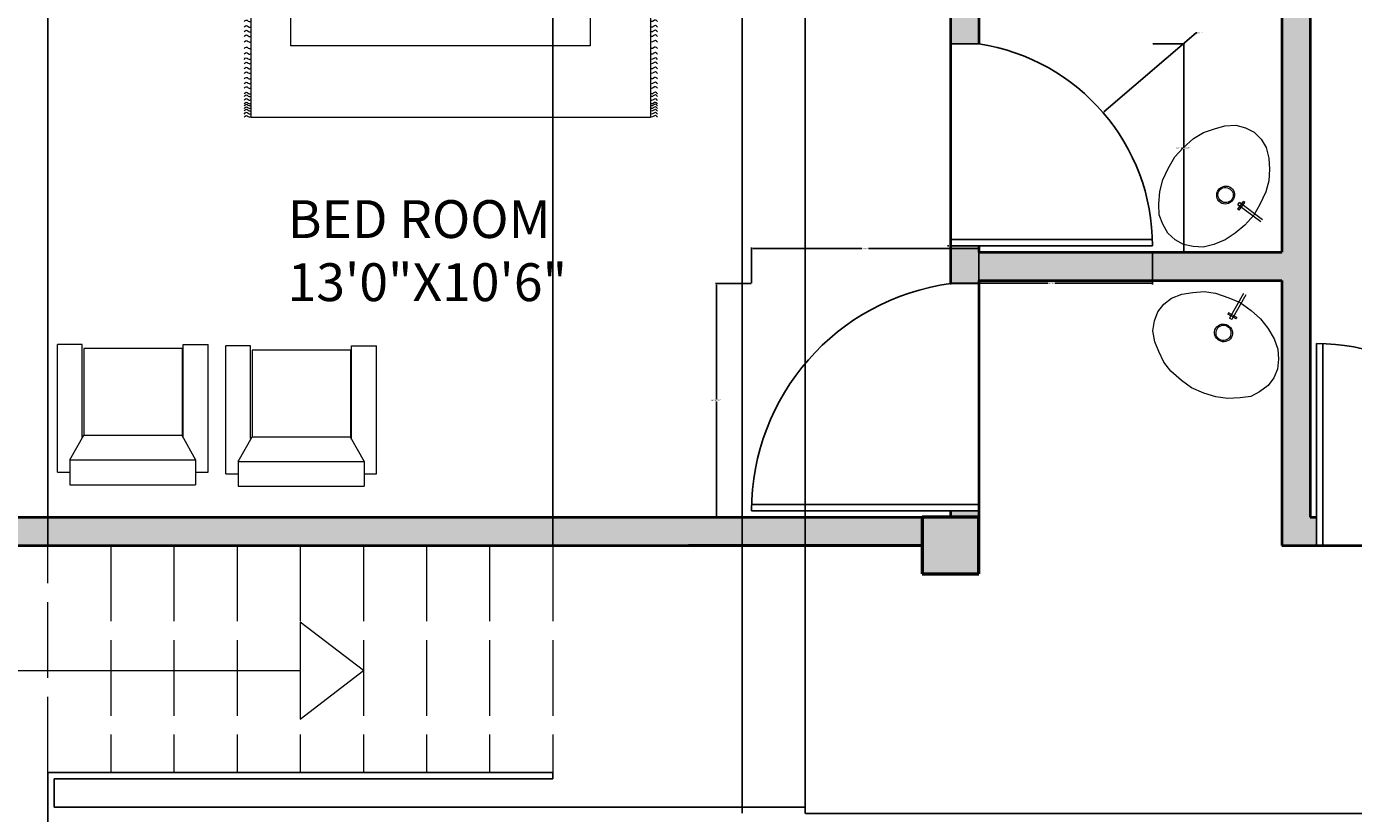
# Model space of a CAD drawing. Units: inches. Extents: x 25176543 to 25177243, y 80295576 to 80296086.
# Tile 3 of 11: x 25176668 to 25176879, y 80295843 to 80295968. Entities that reach past the tile are written whole.
import ezdxf

# ---------------------------------------------------------------- set-up
doc = ezdxf.new("R2010")
doc.units = ezdxf.units.IN
doc.header["$MEASUREMENT"] = 0
doc.linetypes.add('ACAD_ISO02W100', pattern=[15, 12, -3])
for name, color, linetype, lineweight in [('A-ANNO-DIMS', 2, 'Continuous', 18), ('A-ANNO-SYMB', 7, 'Continuous', 18), ('A-AREA-IDEN', 7, 'Continuous', 18), ('A-COLS', 7, 'Continuous', 50), ('A-COLS-PATT', 251, 'Continuous', 13), ('A-DOOR', 3, 'Continuous', 25), ('A-FLOR-FIXT', 8, 'Continuous', 18), ('A-FLOR-STRS', 7, 'Continuous', 25), ('A-FLOR-STRS-OVHD', 7, 'ACAD_ISO02W100', 18), ('A-WALL', 7, 'Continuous', 40), ('A-WALL-PATT', 146, 'Continuous', 13), ('furniture', 31, 'Continuous', 13)]:
    doc.layers.add(name, color=color, linetype=linetype, lineweight=lineweight)
doc.styles.get("Standard").update_dxf_attribs({"font": 'arial.ttf'})
doc.dimstyles.get("Standard").update_dxf_attribs({"dimtxt": 0.18, "dimasz": 0.18, "dimexe": 0.18, "dimexo": 0.0625, "dimgap": 0.09, "dimtad": 0, "dimtih": 1, "dimtoh": 1, "dimdec": 4, "dimzin": 0, "dimdsep": 46, "dimtxsty": 'Standard', "dimcen": 0.09, "dimadec": 0, "dimazin": 0, "dimtfac": 1, "dimtdec": 4, "dimtofl": 0, "dimtmove": 0, "dimatfit": 3, "dimfxl": 1, "dimtolj": 1, "dimtzin": 0, "dimarcsym": 0})

# ---------------------------------------------------------------- blocks, each defined once
blk = doc.blocks.new('BED-DOUBLE-WITH-NIGHTSTANDS')
for p, q in [((5.6, 61.62), (5.6, 51.56)), ((63.65, 61.72), (63.65, 51.66)), ((10.63, 56.59), (0.57, 56.59)), ((68.68, 56.69), (58.62, 56.69)), ((49.39, 52.82), (10.63, 52.82)), ((49.39, 52.82), (58, 46.47)), ((49.44, 52.82), (49.44, 46.47)), ((49.44, 52), (10.63, 52)), ((49.44, 46.47), (58, 46.47)), ((58.05, 34.96), (10.63, 34.96)), ((4.35, 0), (4.35, 26.37)), ((4.35, 26.37), (10.65, 26.37)), ((58.05, 26.37), (67.59, 26.37)), ((67.59, 26.37), (67.59, 0)), ((67.59, 0), (4.35, 0))]:
    blk.add_line(p, q)
for points in [[(0, 50.39), (10.63, 50.5), (10.63, 62.68), (0, 62.58)], [(58.05, 62.68), (58.05, 11.37), (10.63, 11.37), (10.63, 62.68)], [(58.05, 50.5), (68.68, 50.6), (68.68, 62.78), (58.05, 62.68)], [(29.88, 59.98), (29.88, 52.82), (15.98, 52.82), (15.98, 59.98)], [(49.44, 59.98), (49.44, 52.82), (35.55, 52.82), (35.55, 59.98)]]:
    blk.add_lwpolyline(points, close=True)
for centre in [(5.6, 56.59), (63.65, 56.69)]:
    blk.add_circle(centre, 3.92)
for points, knots in [([(3.23, 25.84), (3.32, 25.96), (3.52, 26.2), (3.86, 25.96), (4.14, 25.78), (4.29, 25.89), (4.35, 25.94)], [0, 0, 0, 0, 0.400747, 0.791423, 1.067667, 1.29709, 1.29709, 1.29709, 1.29709]), ([(3.23, 25.06), (3.32, 25.18), (3.52, 25.42), (3.86, 25.18), (4.14, 25.01), (4.29, 25.11), (4.35, 25.16)], [0, 0, 0, 0, 0.400747, 0.791423, 1.067667, 1.29709, 1.29709, 1.29709, 1.29709]), ([(68.71, 25.84), (68.61, 25.96), (68.42, 26.2), (68.08, 25.96), (67.8, 25.78), (67.65, 25.89), (67.58, 25.94)], [0, 0, 0, 0, 0.400747, 0.791423, 1.067667, 1.29709, 1.29709, 1.29709, 1.29709]), ([(68.71, 25.06), (68.61, 25.18), (68.42, 25.42), (68.08, 25.18), (67.8, 25.01), (67.65, 25.11), (67.58, 25.16)], [0, 0, 0, 0, 0.400747, 0.791423, 1.067667, 1.29709, 1.29709, 1.29709, 1.29709]), ([(3.23, 24.24), (3.32, 24.36), (3.52, 24.6), (3.86, 24.36), (4.14, 24.19), (4.29, 24.3), (4.35, 24.34)], [0, 0, 0, 0, 0.400747, 0.791423, 1.067667, 1.29709, 1.29709, 1.29709, 1.29709]), ([(3.23, 23.51), (3.32, 23.63), (3.52, 23.87), (3.86, 23.63), (4.14, 23.46), (4.29, 23.57), (4.35, 23.62)], [0, 0, 0, 0, 0.400747, 0.791423, 1.067667, 1.29709, 1.29709, 1.29709, 1.29709]), ([(68.71, 24.24), (68.61, 24.36), (68.42, 24.6), (68.08, 24.36), (67.8, 24.19), (67.65, 24.3), (67.58, 24.34)], [0, 0, 0, 0, 0.400747, 0.791423, 1.067667, 1.29709, 1.29709, 1.29709, 1.29709]), ([(68.71, 23.51), (68.61, 23.63), (68.42, 23.87), (68.08, 23.63), (67.8, 23.46), (67.65, 23.57), (67.58, 23.62)], [0, 0, 0, 0, 0.400747, 0.791423, 1.067667, 1.29709, 1.29709, 1.29709, 1.29709]), ([(3.23, 22.63), (3.32, 22.75), (3.52, 22.99), (3.86, 22.75), (4.14, 22.58), (4.29, 22.69), (4.35, 22.73)], [0, 0, 0, 0, 0.400747, 0.791423, 1.067667, 1.29709, 1.29709, 1.29709, 1.29709]), ([(3.23, 21.88), (3.32, 22), (3.52, 22.24), (3.86, 22), (4.14, 21.83), (4.29, 21.93), (4.35, 21.98)], [0, 0, 0, 0, 0.400747, 0.791423, 1.067667, 1.29709, 1.29709, 1.29709, 1.29709]), ([(3.23, 21.15), (3.32, 21.27), (3.52, 21.51), (3.86, 21.27), (4.14, 21.1), (4.29, 21.21), (4.35, 21.25)], [0, 0, 0, 0, 0.400747, 0.791423, 1.067667, 1.29709, 1.29709, 1.29709, 1.29709]), ([(68.71, 22.63), (68.61, 22.75), (68.42, 22.99), (68.08, 22.75), (67.8, 22.58), (67.65, 22.69), (67.58, 22.73)], [0, 0, 0, 0, 0.400747, 0.791423, 1.067667, 1.29709, 1.29709, 1.29709, 1.29709]), ([(68.71, 21.88), (68.61, 22), (68.42, 22.24), (68.08, 22), (67.8, 21.83), (67.65, 21.93), (67.58, 21.98)], [0, 0, 0, 0, 0.400747, 0.791423, 1.067667, 1.29709, 1.29709, 1.29709, 1.29709]), ([(68.71, 21.15), (68.61, 21.27), (68.42, 21.51), (68.08, 21.27), (67.8, 21.1), (67.65, 21.21), (67.58, 21.25)], [0, 0, 0, 0, 0.400747, 0.791423, 1.067667, 1.29709, 1.29709, 1.29709, 1.29709]), ([(3.23, 20.27), (3.32, 20.39), (3.52, 20.63), (3.86, 20.39), (4.14, 20.22), (4.29, 20.32), (4.35, 20.37)], [0, 0, 0, 0, 0.400747, 0.791423, 1.067667, 1.29709, 1.29709, 1.29709, 1.29709]), ([(3.23, 19.23), (3.32, 19.35), (3.52, 19.59), (3.86, 19.35), (4.14, 19.18), (4.29, 19.29), (4.35, 19.33)], [0, 0, 0, 0, 0.400747, 0.791423, 1.067667, 1.29709, 1.29709, 1.29709, 1.29709]), ([(68.71, 20.27), (68.61, 20.39), (68.42, 20.63), (68.08, 20.39), (67.8, 20.22), (67.65, 20.32), (67.58, 20.37)], [0, 0, 0, 0, 0.400747, 0.791423, 1.067667, 1.29709, 1.29709, 1.29709, 1.29709]), ([(68.71, 19.23), (68.61, 19.35), (68.42, 19.59), (68.08, 19.35), (67.8, 19.18), (67.65, 19.29), (67.58, 19.33)], [0, 0, 0, 0, 0.400747, 0.791423, 1.067667, 1.29709, 1.29709, 1.29709, 1.29709]), ([(3.23, 18.35), (3.32, 18.47), (3.52, 18.71), (3.86, 18.47), (4.14, 18.3), (4.29, 18.4), (4.35, 18.45)], [0, 0, 0, 0, 0.400747, 0.791423, 1.067667, 1.29709, 1.29709, 1.29709, 1.29709]), ([(3.23, 17.53), (3.32, 17.65), (3.52, 17.89), (3.86, 17.65), (4.14, 17.48), (4.29, 17.59), (4.35, 17.64)], [0, 0, 0, 0, 0.400747, 0.791423, 1.067667, 1.29709, 1.29709, 1.29709, 1.29709]), ([(3.23, 16.76), (3.32, 16.88), (3.52, 17.12), (3.86, 16.88), (4.14, 16.7), (4.29, 16.81), (4.35, 16.86)], [0, 0, 0, 0, 0.400747, 0.791423, 1.067667, 1.29709, 1.29709, 1.29709, 1.29709]), ([(68.71, 18.35), (68.61, 18.47), (68.42, 18.71), (68.08, 18.47), (67.8, 18.3), (67.65, 18.4), (67.58, 18.45)], [0, 0, 0, 0, 0.400747, 0.791423, 1.067667, 1.29709, 1.29709, 1.29709, 1.29709]), ([(68.71, 17.53), (68.61, 17.65), (68.42, 17.89), (68.08, 17.65), (67.8, 17.48), (67.65, 17.59), (67.58, 17.64)], [0, 0, 0, 0, 0.400747, 0.791423, 1.067667, 1.29709, 1.29709, 1.29709, 1.29709]), ([(68.71, 16.76), (68.61, 16.88), (68.42, 17.12), (68.08, 16.88), (67.8, 16.7), (67.65, 16.81), (67.58, 16.86)], [0, 0, 0, 0, 0.400747, 0.791423, 1.067667, 1.29709, 1.29709, 1.29709, 1.29709]), ([(3.23, 15.94), (3.32, 16.06), (3.52, 16.3), (3.86, 16.06), (4.14, 15.89), (4.29, 16), (4.35, 16.04)], [0, 0, 0, 0, 0.400747, 0.791423, 1.067667, 1.29709, 1.29709, 1.29709, 1.29709]), ([(3.23, 15.21), (3.32, 15.33), (3.52, 15.57), (3.86, 15.33), (4.14, 15.16), (4.29, 15.27), (4.35, 15.32)], [0, 0, 0, 0, 0.400747, 0.791423, 1.067667, 1.29709, 1.29709, 1.29709, 1.29709]), ([(68.71, 15.94), (68.61, 16.06), (68.42, 16.3), (68.08, 16.06), (67.8, 15.89), (67.65, 16), (67.58, 16.04)], [0, 0, 0, 0, 0.400747, 0.791423, 1.067667, 1.29709, 1.29709, 1.29709, 1.29709]), ([(68.71, 15.21), (68.61, 15.33), (68.42, 15.57), (68.08, 15.33), (67.8, 15.16), (67.65, 15.27), (67.58, 15.32)], [0, 0, 0, 0, 0.400747, 0.791423, 1.067667, 1.29709, 1.29709, 1.29709, 1.29709]), ([(3.23, 14.33), (3.32, 14.45), (3.52, 14.69), (3.86, 14.45), (4.14, 14.28), (4.29, 14.38), (4.35, 14.43)], [0, 0, 0, 0, 0.400747, 0.791423, 1.067667, 1.29709, 1.29709, 1.29709, 1.29709]), ([(3.23, 13.58), (3.32, 13.7), (3.52, 13.94), (3.86, 13.7), (4.14, 13.53), (4.29, 13.63), (4.35, 13.68)], [0, 0, 0, 0, 0.400747, 0.791423, 1.067667, 1.29709, 1.29709, 1.29709, 1.29709]), ([(3.23, 12.85), (3.32, 12.97), (3.52, 13.21), (3.86, 12.97), (4.14, 12.8), (4.29, 12.9), (4.35, 12.95)], [0, 0, 0, 0, 0.400747, 0.791423, 1.067667, 1.29709, 1.29709, 1.29709, 1.29709]), ([(68.71, 14.33), (68.61, 14.45), (68.42, 14.69), (68.08, 14.45), (67.8, 14.28), (67.65, 14.38), (67.58, 14.43)], [0, 0, 0, 0, 0.400747, 0.791423, 1.067667, 1.29709, 1.29709, 1.29709, 1.29709]), ([(68.71, 13.58), (68.61, 13.7), (68.42, 13.94), (68.08, 13.7), (67.8, 13.53), (67.65, 13.63), (67.58, 13.68)], [0, 0, 0, 0, 0.400747, 0.791423, 1.067667, 1.29709, 1.29709, 1.29709, 1.29709]), ([(68.71, 12.85), (68.61, 12.97), (68.42, 13.21), (68.08, 12.97), (67.8, 12.8), (67.65, 12.9), (67.58, 12.95)], [0, 0, 0, 0, 0.400747, 0.791423, 1.067667, 1.29709, 1.29709, 1.29709, 1.29709]), ([(3.23, 11.97), (3.32, 12.09), (3.52, 12.33), (3.86, 12.09), (4.14, 11.92), (4.29, 12.02), (4.35, 12.07)], [0, 0, 0, 0, 0.400747, 0.791423, 1.067667, 1.29709, 1.29709, 1.29709, 1.29709]), ([(3.23, 10.93), (3.32, 11.05), (3.52, 11.29), (3.86, 11.05), (4.14, 10.88), (4.29, 10.99), (4.35, 11.03)], [0, 0, 0, 0, 0.400747, 0.791423, 1.067667, 1.29709, 1.29709, 1.29709, 1.29709]), ([(68.71, 11.97), (68.61, 12.09), (68.42, 12.33), (68.08, 12.09), (67.8, 11.92), (67.65, 12.02), (67.58, 12.07)], [0, 0, 0, 0, 0.400747, 0.791423, 1.067667, 1.29709, 1.29709, 1.29709, 1.29709]), ([(68.71, 10.93), (68.61, 11.05), (68.42, 11.29), (68.08, 11.05), (67.8, 10.88), (67.65, 10.99), (67.58, 11.03)], [0, 0, 0, 0, 0.400747, 0.791423, 1.067667, 1.29709, 1.29709, 1.29709, 1.29709]), ([(3.23, 10.05), (3.32, 10.17), (3.52, 10.41), (3.86, 10.17), (4.14, 10), (4.29, 10.1), (4.35, 10.15)], [0, 0, 0, 0, 0.400747, 0.791423, 1.067667, 1.29709, 1.29709, 1.29709, 1.29709]), ([(3.23, 9.23), (3.32, 9.35), (3.52, 9.59), (3.86, 9.35), (4.14, 9.18), (4.29, 9.29), (4.35, 9.34)], [0, 0, 0, 0, 0.400747, 0.791423, 1.067667, 1.29709, 1.29709, 1.29709, 1.29709]), ([(3.23, 8.54), (3.32, 8.66), (3.52, 8.9), (3.86, 8.66), (4.14, 8.49), (4.29, 8.6), (4.35, 8.65)], [0, 0, 0, 0, 0.400747, 0.791423, 1.067667, 1.29709, 1.29709, 1.29709, 1.29709]), ([(68.71, 10.05), (68.61, 10.17), (68.42, 10.41), (68.08, 10.17), (67.8, 10), (67.65, 10.1), (67.58, 10.15)], [0, 0, 0, 0, 0.400747, 0.791423, 1.067667, 1.29709, 1.29709, 1.29709, 1.29709]), ([(68.71, 9.23), (68.61, 9.35), (68.42, 9.59), (68.08, 9.35), (67.8, 9.18), (67.65, 9.29), (67.58, 9.34)], [0, 0, 0, 0, 0.400747, 0.791423, 1.067667, 1.29709, 1.29709, 1.29709, 1.29709]), ([(68.71, 8.54), (68.61, 8.66), (68.42, 8.9), (68.08, 8.66), (67.8, 8.49), (67.65, 8.6), (67.58, 8.65)], [0, 0, 0, 0, 0.400747, 0.791423, 1.067667, 1.29709, 1.29709, 1.29709, 1.29709]), ([(3.23, 7.73), (3.32, 7.85), (3.52, 8.09), (3.86, 7.85), (4.14, 7.68), (4.29, 7.78), (4.35, 7.83)], [0, 0, 0, 0, 0.400747, 0.791423, 1.067667, 1.29709, 1.29709, 1.29709, 1.29709]), ([(3.23, 7), (3.32, 7.12), (3.52, 7.36), (3.86, 7.12), (4.14, 6.95), (4.29, 7.05), (4.35, 7.1)], [0, 0, 0, 0, 0.400747, 0.791423, 1.067667, 1.29709, 1.29709, 1.29709, 1.29709]), ([(3.23, 6.12), (3.32, 6.24), (3.52, 6.48), (3.86, 6.24), (4.14, 6.07), (4.29, 6.17), (4.35, 6.22)], [0, 0, 0, 0, 0.400747, 0.791423, 1.067667, 1.29709, 1.29709, 1.29709, 1.29709]), ([(68.71, 7.73), (68.61, 7.85), (68.42, 8.09), (68.08, 7.85), (67.8, 7.68), (67.65, 7.78), (67.58, 7.83)], [0, 0, 0, 0, 0.400747, 0.791423, 1.067667, 1.29709, 1.29709, 1.29709, 1.29709]), ([(68.71, 7), (68.61, 7.12), (68.42, 7.36), (68.08, 7.12), (67.8, 6.95), (67.65, 7.05), (67.58, 7.1)], [0, 0, 0, 0, 0.400747, 0.791423, 1.067667, 1.29709, 1.29709, 1.29709, 1.29709]), ([(68.71, 6.12), (68.61, 6.24), (68.42, 6.48), (68.08, 6.24), (67.8, 6.07), (67.65, 6.17), (67.58, 6.22)], [0, 0, 0, 0, 0.400747, 0.791423, 1.067667, 1.29709, 1.29709, 1.29709, 1.29709]), ([(3.23, 5.36), (3.32, 5.49), (3.52, 5.73), (3.86, 5.49), (4.14, 5.31), (4.29, 5.42), (4.35, 5.47)], [0, 0, 0, 0, 0.400747, 0.791423, 1.067667, 1.29709, 1.29709, 1.29709, 1.29709]), ([(3.23, 4.64), (3.32, 4.76), (3.52, 5), (3.86, 4.76), (4.14, 4.59), (4.29, 4.69), (4.35, 4.74)], [0, 0, 0, 0, 0.400747, 0.791423, 1.067667, 1.29709, 1.29709, 1.29709, 1.29709]), ([(68.71, 5.36), (68.61, 5.49), (68.42, 5.73), (68.08, 5.49), (67.8, 5.31), (67.65, 5.42), (67.58, 5.47)], [0, 0, 0, 0, 0.400747, 0.791423, 1.067667, 1.29709, 1.29709, 1.29709, 1.29709]), ([(68.71, 4.64), (68.61, 4.76), (68.42, 5), (68.08, 4.76), (67.8, 4.59), (67.66, 4.69), (67.59, 4.73)], [0, 0, 0, 0, 0.400747, 0.791423, 1.067667, 1.283686, 1.283686, 1.283686, 1.283686]), ([(3.23, 3.75), (3.32, 3.88), (3.52, 4.12), (3.86, 3.88), (4.14, 3.7), (4.29, 3.81), (4.35, 3.86)], [0, 0, 0, 0, 0.400747, 0.791423, 1.067667, 1.29709, 1.29709, 1.29709, 1.29709]), ([(3.23, 3.33), (3.32, 3.45), (3.52, 3.7), (3.86, 3.44), (4.14, 3.27), (4.29, 3.38), (4.35, 3.43)], [0, 0, 0, 0, 0.407265, 0.802015, 1.07826, 1.307683, 1.307683, 1.307683, 1.307683]), ([(3.23, 2.76), (3.32, 2.88), (3.52, 3.12), (3.86, 2.88), (4.14, 2.71), (4.29, 2.81), (4.35, 2.86)], [0, 0, 0, 0, 0.400747, 0.791423, 1.067667, 1.29709, 1.29709, 1.29709, 1.29709]), ([(3.23, 2.18), (3.32, 2.31), (3.52, 2.55), (3.86, 2.31), (4.14, 2.13), (4.29, 2.24), (4.35, 2.29)], [0, 0, 0, 0, 0.400747, 0.791423, 1.067667, 1.29709, 1.29709, 1.29709, 1.29709]), ([(3.23, 1.88), (3.32, 2), (3.52, 2.24), (3.86, 2), (4.14, 1.82), (4.29, 1.93), (4.35, 1.98)], [0, 0, 0, 0, 0.400747, 0.791423, 1.067667, 1.29709, 1.29709, 1.29709, 1.29709]), ([(68.71, 3.75), (68.61, 3.88), (68.42, 4.11), (68.08, 3.88), (67.8, 3.7), (67.66, 3.81), (67.59, 3.85)], [0, 0, 0, 0, 0.400747, 0.791423, 1.067667, 1.283686, 1.283686, 1.283686, 1.283686]), ([(68.71, 3.33), (68.61, 3.45), (68.42, 3.69), (68.08, 3.45), (67.8, 3.27), (67.66, 3.38), (67.59, 3.42)], [0, 0, 0, 0, 0.402903, 0.794912, 1.071156, 1.287177, 1.287177, 1.287177, 1.287177]), ([(68.71, 2.73), (68.61, 2.85), (68.42, 3.09), (68.08, 2.85), (67.8, 2.68), (67.66, 2.78), (67.59, 2.82)], [0, 0, 0, 0, 0.400747, 0.791423, 1.067667, 1.283686, 1.283686, 1.283686, 1.283686]), ([(68.71, 2.16), (68.61, 2.28), (68.42, 2.52), (68.08, 2.28), (67.8, 2.11), (67.66, 2.21), (67.59, 2.25)], [0, 0, 0, 0, 0.400747, 0.791423, 1.067667, 1.283686, 1.283686, 1.283686, 1.283686]), ([(68.71, 1.85), (68.61, 1.97), (68.42, 2.21), (68.08, 1.97), (67.8, 1.8), (67.66, 1.9), (67.59, 1.94)], [0, 0, 0, 0, 0.400747, 0.791423, 1.067667, 1.283686, 1.283686, 1.283686, 1.283686]), ([(3.23, 1.46), (3.32, 1.58), (3.52, 1.82), (3.86, 1.58), (4.14, 1.41), (4.29, 1.51), (4.35, 1.56)], [0, 0, 0, 0, 0.400747, 0.791423, 1.067667, 1.29709, 1.29709, 1.29709, 1.29709]), ([(3.23, 1.06), (3.32, 1.18), (3.52, 1.42), (3.86, 1.18), (4.14, 1.01), (4.29, 1.11), (4.35, 1.16)], [0, 0, 0, 0, 0.400747, 0.791423, 1.067667, 1.29709, 1.29709, 1.29709, 1.29709]), ([(3.23, 0.57), (3.32, 0.7), (3.52, 0.94), (3.86, 0.7), (4.14, 0.52), (4.29, 0.63), (4.35, 0.68)], [0, 0, 0, 0, 0.400747, 0.791423, 1.067667, 1.29709, 1.29709, 1.29709, 1.29709]), ([(3.23, 0.07), (3.32, 0.19), (3.52, 0.43), (3.86, 0.19), (4.14, 0.02), (4.29, 0.13), (4.35, 0.18)], [0, 0, 0, 0, 0.400747, 0.791423, 1.067667, 1.29709, 1.29709, 1.29709, 1.29709]), ([(68.71, 1.43), (68.61, 1.55), (68.42, 1.79), (68.08, 1.55), (67.8, 1.38), (67.65, 1.48), (67.58, 1.53)], [0, 0, 0, 0, 0.400747, 0.791423, 1.067667, 1.29709, 1.29709, 1.29709, 1.29709]), ([(68.71, 1.03), (68.61, 1.15), (68.42, 1.39), (68.08, 1.15), (67.8, 0.98), (67.65, 1.09), (67.58, 1.13)], [0, 0, 0, 0, 0.400747, 0.791423, 1.067667, 1.29709, 1.29709, 1.29709, 1.29709]), ([(68.71, 0.55), (68.61, 0.67), (68.42, 0.91), (68.08, 0.67), (67.8, 0.49), (67.65, 0.6), (67.58, 0.65)], [0, 0, 0, 0, 0.400747, 0.791423, 1.067667, 1.29709, 1.29709, 1.29709, 1.29709]), ([(68.71, 0.07), (68.61, 0.19), (68.42, 0.43), (68.08, 0.19), (67.8, 0.02), (67.65, 0.13), (67.58, 0.18)], [0, 0, 0, 0, 0.400747, 0.791423, 1.067667, 1.29709, 1.29709, 1.29709, 1.29709])]:
    blk.add_open_spline(points, degree=3, knots=knots)
blk = doc.blocks.new('LOUNGE-CHAIR')
for p, q in [((0, 1.96), (0, 22.23)), ((3.92, 22.23), (0, 22.23)), ((3.92, 7.54), (3.92, 22.23)), ((19.74, 21.58), (19.74, 7.85)), ((19.93, 7.41), (19.93, 22.23)), ((19.93, 22.23), (23.85, 22.23)), ((23.85, 1.96), (23.85, 22.23)), ((1.96, 3.92), (4.17, 7.85)), ((19.68, 7.85), (21.89, 3.92)), ((1.96, 3.92), (21.89, 3.92)), ((1.96, 3.92), (1.96, 0)), ((21.89, 3.92), (21.89, 0)), ((0, 1.96), (1.96, 1.96)), ((1.96, 0), (21.89, 0)), ((21.89, 1.96), (23.85, 1.96))]:
    blk.add_line(p, q)
blk.add_lwpolyline([(19.93, 21.58), (4.17, 21.58), (4.17, 7.85), (19.74, 7.85)])
blk = doc.blocks.new('WASH-BASIN')
for p, q in [((12.49, 6.73), (12.74, 7.07)), ((13.61, 7.11), (13.41, 7.26)), ((12.71, 5.89), (12.51, 6.04))]:
    blk.add_line(p, q)
for points in [[(2.54, 1.2), (1.42, 2.23), (0.6, 3.68), (0.01, 5.16), (0, 6.84), (0.12, 8.85), (0.63, 10.67), (1.44, 12.48), (2.49, 14.33), (3.84, 15.74), (5.48, 17.25), (7.03, 18.21), (8.81, 18.78), (10.43, 19.26), (12.16, 19.34), (13.73, 18.91), (15.1, 18.22), (16.17, 17.11), (16.98, 15.79), (17.41, 14.1), (17.49, 12.37), (17.4, 10.55), (16.94, 8.79), (15.98, 6.78), (15.03, 5.07), (13.58, 3.52), (12.09, 2.21), (10.49, 1.19), (8.68, 0.43), (7, 0), (5.41, 0.12), (3.86, 0.43)], [(12.59, 6.87), (12.59, 6.87)], [(13.33, 7.16), (13.33, 7.16)], [(12.43, 5.94), (12.43, 5.94)]]:
    blk.add_lwpolyline(points, close=True)
for points in [[(16.15, 4.03), (12.49, 6.73), (12.49, 6.73)], [(12.51, 6.04), (13.41, 7.26), (13.41, 7.26)], [(12.71, 5.89), (13.61, 7.11), (13.61, 7.11)], [(16.4, 4.37), (12.74, 7.07), (12.74, 7.07)]]:
    blk.add_lwpolyline(points)
for points in [[(9.72, 7.1), (10.34, 6.65), (11.21, 6.84), (11.66, 7.45), (11.66, 7.45), (12.11, 8.06), (12.04, 8.96), (11.43, 9.41), (11.43, 9.41), (10.75, 9.91), (9.87, 9.71), (9.42, 9.1), (9.42, 9.1), (8.97, 8.49), (9.05, 7.6), (9.72, 7.1)], [(9.88, 7.3), (10.35, 6.95), (11.12, 7.01), (11.53, 7.55), (11.53, 7.55), (11.93, 8.1), (11.75, 8.85), (11.28, 9.2), (11.28, 9.2), (10.73, 9.6), (9.96, 9.55), (9.56, 9), (9.56, 9), (9.16, 8.46), (9.33, 7.7), (9.88, 7.3)]]:
    blk.add_open_spline(points, degree=3, knots=[0, 0, 0, 0, 0.0625, 0.0625, 0.0625, 0.062501, 0.125, 0.125, 0.125, 0.125001, 0.1875, 0.1875, 0.1875, 0.187501, 1, 1, 1, 1])
blk = doc.blocks.new('DOOR-32IN')
for p, q in [((0, 1), (0, 33)), ((0, 33), (4.5, 33)), ((32, 2), (0, 2)), ((0, 0), (0, 1)), ((0, 1), (32, 1)), ((32, 1), (0, 1))]:
    blk.add_line(p, q)
blk.add_arc((-0.37, 1), 32.37, 0, 81.3499)
blk = doc.blocks.new('DOOR-36IN')
for p, q in [((36, 37), (31.5, 37)), ((36, 1), (36, 37)), ((0, 2), (36, 2)), ((36, 1), (0, 1)), ((0, 1), (36, 1)), ((36, 0), (36, 1))]:
    blk.add_line(p, q)
blk.add_arc((36.32, 1), 36.32, 97.6281, 180)
blk = doc.blocks.new('COLUMN-9IN-SQ')
for p, q in [((9, 9), (0, 9)), ((0, 9), (0, 0)), ((9, 0), (9, 9)), ((0, 0), (9, 0))]:
    blk.add_line(p, q)
blk = doc.blocks.new('*D38')
at = {"layer": 'A-ANNO-DIMS', "color": 0, "lineweight": -2, "transparency": 16777216}
for p, q in [((25176783.24, 80295927.3), (25176777.57, 80295927.3)), ((25176777.75, 80295927.12), (25176777.75, 80295908.99)), ((25176777.75, 80295890.48), (25176777.75, 80295908.62)), ((25176783.24, 80295890.3), (25176777.57, 80295890.3))]:
    blk.add_line(p, q, dxfattribs=at)
at = {"layer": 'A-ANNO-DIMS', "color": 0, "transparency": 16777216}
for points in [[(25176777.72, 80295927.12), (25176777.78, 80295927.12), (25176777.75, 80295927.3)], [(25176777.72, 80295890.48), (25176777.78, 80295890.48), (25176777.75, 80295890.3)]]:
    blk.add_solid(points, dxfattribs=at)
at = {"layer": 'Defpoints', "color": 0, "transparency": 16777216}
for p in [(25176777.75, 80295927.3), (25176783.3, 80295927.3), (25176783.3, 80295890.3)]:
    blk.add_point(p, dxfattribs=at)
at = {"layer": 'A-ANNO-DIMS', "color": 0, "transparency": 16777216, "insert": (25176777.75, 80295908.8), "char_height": 0.18, "attachment_point": 5}
blk.add_mtext('\\A1;DOOR 37 TYP.', dxfattribs=at)
blk = doc.blocks.new('*D39')
at = {"layer": 'A-ANNO-DIMS', "color": 0, "lineweight": -2, "transparency": 16777216}
for p, q in [((25176783.3, 80295927.36), (25176783.3, 80295933.03)), ((25176783.48, 80295932.85), (25176800.77, 80295932.85)), ((25176819.12, 80295932.85), (25176801.83, 80295932.85)), ((25176819.3, 80295927.36), (25176819.3, 80295933.03))]:
    blk.add_line(p, q, dxfattribs=at)
at = {"layer": 'A-ANNO-DIMS', "color": 0, "transparency": 16777216}
for points in [[(25176783.48, 80295932.88), (25176783.48, 80295932.82), (25176783.3, 80295932.85)], [(25176819.12, 80295932.88), (25176819.12, 80295932.82), (25176819.3, 80295932.85)]]:
    blk.add_solid(points, dxfattribs=at)
at = {"layer": 'Defpoints', "color": 0, "transparency": 16777216}
for p in [(25176819.3, 80295932.85), (25176783.3, 80295927.3), (25176819.3, 80295927.3)]:
    blk.add_point(p, dxfattribs=at)
at = {"layer": 'A-ANNO-DIMS', "color": 0, "transparency": 16777216, "insert": (25176801.3, 80295932.85), "char_height": 0.18, "attachment_point": 5}
blk.add_mtext('\\A1;36 TYP.', dxfattribs=at)
blk = doc.blocks.new('*D40')
at = {"layer": 'A-ANNO-DIMS', "color": 0, "lineweight": -2, "transparency": 16777216}
for p, q in [((25176846.86, 80295965.3), (25176851.93, 80295965.3)), ((25176851.75, 80295965.12), (25176851.75, 80295948.99)), ((25176851.75, 80295932.48), (25176851.75, 80295948.62)), ((25176846.86, 80295932.3), (25176851.93, 80295932.3))]:
    blk.add_line(p, q, dxfattribs=at)
at = {"layer": 'A-ANNO-DIMS', "color": 0, "transparency": 16777216}
for points in [[(25176851.72, 80295965.12), (25176851.78, 80295965.12), (25176851.75, 80295965.3)], [(25176851.72, 80295932.48), (25176851.78, 80295932.48), (25176851.75, 80295932.3)]]:
    blk.add_solid(points, dxfattribs=at)
at = {"layer": 'Defpoints', "color": 0, "transparency": 16777216}
for p in [(25176846.8, 80295965.3), (25176851.75, 80295965.3), (25176846.8, 80295932.3)]:
    blk.add_point(p, dxfattribs=at)
at = {"layer": 'A-ANNO-DIMS', "color": 0, "transparency": 16777216, "insert": (25176851.75, 80295948.8), "char_height": 0.18, "attachment_point": 5}
blk.add_mtext('\\A1;BATH DOOR 33 TYP.', dxfattribs=at)
blk = doc.blocks.new('*D41')
at = {"layer": 'A-ANNO-DIMS', "color": 0, "lineweight": -2, "transparency": 16777216}
for p, q in [((25176814.8, 80295932.24), (25176814.8, 80295927.17)), ((25176846.8, 80295932.24), (25176846.8, 80295927.17)), ((25176814.98, 80295927.35), (25176830.27, 80295927.35)), ((25176846.62, 80295927.35), (25176831.33, 80295927.35))]:
    blk.add_line(p, q, dxfattribs=at)
at = {"layer": 'A-ANNO-DIMS', "color": 0, "transparency": 16777216}
for points in [[(25176814.98, 80295927.38), (25176814.98, 80295927.32), (25176814.8, 80295927.35)], [(25176846.62, 80295927.38), (25176846.62, 80295927.32), (25176846.8, 80295927.35)]]:
    blk.add_solid(points, dxfattribs=at)
at = {"layer": 'Defpoints', "color": 0, "transparency": 16777216}
for p in [(25176814.8, 80295932.3), (25176846.8, 80295932.3), (25176846.8, 80295927.35)]:
    blk.add_point(p, dxfattribs=at)
at = {"layer": 'A-ANNO-DIMS', "color": 0, "transparency": 16777216, "insert": (25176830.8, 80295927.35), "char_height": 0.18, "attachment_point": 5}
blk.add_mtext('\\A1;32 TYP.', dxfattribs=at)
blk = doc.blocks.new('*D48')
at = {"layer": 'A-ANNO-DIMS', "color": 0, "lineweight": -2, "transparency": 16777216}
for p, q in [((25176625.3, 80295890.36), (25176625.3, 80296052.23)), ((25176625.48, 80296052.05), (25176875.16, 80296052.05)), ((25177125.62, 80296052.05), (25176875.95, 80296052.05)), ((25177125.8, 80296025.36), (25177125.8, 80296052.23))]:
    blk.add_line(p, q, dxfattribs=at)
at = {"layer": 'A-ANNO-DIMS', "color": 0, "transparency": 16777216}
for points in [[(25176625.48, 80296052.08), (25176625.48, 80296052.02), (25176625.3, 80296052.05)], [(25177125.62, 80296052.08), (25177125.62, 80296052.02), (25177125.8, 80296052.05)]]:
    blk.add_solid(points, dxfattribs=at)
at = {"layer": 'Defpoints', "color": 0, "transparency": 16777216}
for p in [(25177125.8, 80296052.05), (25177125.8, 80296025.3), (25176625.3, 80295890.3)]:
    blk.add_point(p, dxfattribs=at)
at = {"layer": 'A-ANNO-DIMS', "color": 0, "transparency": 16777216, "insert": (25176875.55, 80296052.05), "char_height": 0.18, "attachment_point": 5}
blk.add_mtext('\\A1;500.5', dxfattribs=at)
blk = doc.blocks.new('*D73')
at = {"layer": 'A-ANNO-DIMS', "color": 0, "lineweight": -2, "transparency": 16777216}
for p, q in [((25176791.86, 80295843.3), (25177152.73, 80295843.3)), ((25177152.55, 80295843.12), (25177152.55, 80295825.48)), ((25177152.55, 80295807.48), (25177152.55, 80295825.12)), ((25176791.86, 80295807.3), (25177152.73, 80295807.3))]:
    blk.add_line(p, q, dxfattribs=at)
at = {"layer": 'A-ANNO-DIMS', "color": 0, "transparency": 16777216}
for points in [[(25177152.52, 80295843.12), (25177152.58, 80295843.12), (25177152.55, 80295843.3)], [(25177152.52, 80295807.48), (25177152.58, 80295807.48), (25177152.55, 80295807.3)]]:
    blk.add_solid(points, dxfattribs=at)
at = {"layer": 'Defpoints', "color": 0, "transparency": 16777216}
for p in [(25176791.8, 80295843.3), (25177152.55, 80295843.3), (25176791.8, 80295807.3)]:
    blk.add_point(p, dxfattribs=at)
at = {"layer": 'A-ANNO-DIMS', "color": 0, "transparency": 16777216, "insert": (25177152.55, 80295825.3), "char_height": 0.18, "attachment_point": 5}
blk.add_mtext('\\A1;36', dxfattribs=at)
blk = doc.blocks.new('*D74')
at = {"layer": 'A-ANNO-DIMS', "color": 0, "lineweight": -2, "transparency": 16777216}
for p, q in [((25176671.8, 80295885.86), (25176671.8, 80296052.23)), ((25176671.98, 80296052.05), (25176711.58, 80296052.05)), ((25176751.62, 80296052.05), (25176712.02, 80296052.05)), ((25176751.8, 80295885.86), (25176751.8, 80296052.23))]:
    blk.add_line(p, q, dxfattribs=at)
at = {"layer": 'A-ANNO-DIMS', "color": 0, "transparency": 16777216}
for points in [[(25176671.98, 80296052.08), (25176671.98, 80296052.02), (25176671.8, 80296052.05)], [(25176751.62, 80296052.08), (25176751.62, 80296052.02), (25176751.8, 80296052.05)]]:
    blk.add_solid(points, dxfattribs=at)
at = {"layer": 'Defpoints', "color": 0, "transparency": 16777216}
for p in [(25176751.8, 80296052.05), (25176671.8, 80295885.8), (25176751.8, 80295885.8)]:
    blk.add_point(p, dxfattribs=at)
at = {"layer": 'A-ANNO-DIMS', "color": 0, "transparency": 16777216, "insert": (25176711.8, 80296052.05), "char_height": 0.18, "attachment_point": 5}
blk.add_mtext('\\A1;80', dxfattribs=at)
blk = doc.blocks.new('*D75')
at = {"layer": 'A-ANNO-DIMS', "color": 0, "lineweight": -2, "transparency": 16777216}
for p, q in [((25176781.8, 80295843.36), (25176781.8, 80296052.23)), ((25176781.98, 80296052.05), (25176786.59, 80296052.05)), ((25176791.62, 80296052.05), (25176787.01, 80296052.05)), ((25176791.8, 80295843.36), (25176791.8, 80296052.23))]:
    blk.add_line(p, q, dxfattribs=at)
at = {"layer": 'A-ANNO-DIMS', "color": 0, "transparency": 16777216}
for points in [[(25176781.98, 80296052.08), (25176781.98, 80296052.02), (25176781.8, 80296052.05)], [(25176791.62, 80296052.08), (25176791.62, 80296052.02), (25176791.8, 80296052.05)]]:
    blk.add_solid(points, dxfattribs=at)
at = {"layer": 'Defpoints', "color": 0, "transparency": 16777216}
for p in [(25176791.8, 80296052.05), (25176781.8, 80295843.3), (25176791.8, 80295843.3)]:
    blk.add_point(p, dxfattribs=at)
at = {"layer": 'A-ANNO-DIMS', "color": 0, "transparency": 16777216, "insert": (25176786.8, 80296052.05), "char_height": 0.18, "attachment_point": 5}
blk.add_mtext('\\A1;10', dxfattribs=at)
blk = doc.blocks.new('*D77')
at = {"layer": 'A-ANNO-DIMS', "color": 0, "lineweight": -2, "transparency": 16777216}
for p, q in [((25176853.71, 80295967.06), (25176839.12, 80295954.52)), ((25176853.89, 80295967.06), (25176853.71, 80295967.06)), ((25176814.34, 80295933.3), (25176814.52, 80295933.3)), ((25176814.43, 80295933.21), (25176814.43, 80295933.39))]:
    blk.add_line(p, q, dxfattribs=at)
at = {"layer": 'A-ANNO-DIMS', "color": 0, "transparency": 16777216}
blk.add_solid([(25176839.1, 80295954.54), (25176839.14, 80295954.49), (25176838.98, 80295954.4)], dxfattribs=at)
at = {"layer": 'Defpoints', "color": 0, "transparency": 16777216}
for p in [(25176838.98, 80295954.4), (25176814.43, 80295933.3)]:
    blk.add_point(p, dxfattribs=at)
at = {"layer": 'A-ANNO-DIMS', "color": 0, "transparency": 16777216, "insert": (25176854.37, 80295967.06), "char_height": 0.18, "attachment_point": 5}
blk.add_mtext('\\A1;R32.37', dxfattribs=at)

msp = doc.modelspace()

# ---------------------------------------------------------------- hatches: boundary and pattern name
at = {"layer": 'A-COLS-PATT'}
h = msp.add_hatch(color=256, dxfattribs=at)
h.dxf.hatch_style = 1
h.paths.add_polyline_path([(25176658.8016, 80296025.3022), (25176649.8016, 80296025.3022), (25176649.8016, 80296016.3022), (25176658.8016, 80296016.3022)])
h.paths.add_polyline_path([(25176819.3016, 80296025.3022), (25176810.3016, 80296025.3022), (25176810.3016, 80296016.3022), (25176819.3016, 80296016.3022)])
h.paths.add_polyline_path([(25176876.3016, 80296025.3022), (25176867.3016, 80296025.3022), (25176867.3016, 80296016.3022), (25176876.3016, 80296016.3022)])
h.paths.add_polyline_path([(25177013.3016, 80296025.3022), (25177004.3016, 80296025.3022), (25177004.3016, 80296016.3022), (25177013.3016, 80296016.3022)])
h.paths.add_polyline_path([(25176819.3016, 80295890.3022), (25176810.3016, 80295890.3022), (25176810.3016, 80295881.3022), (25176819.3016, 80295881.3022)])
h.paths.add_polyline_path([(25176658.8016, 80295890.3022), (25176649.8016, 80295890.3022), (25176649.8016, 80295881.3022), (25176658.8016, 80295881.3022)])
h.paths.add_polyline_path([(25177125.8016, 80296025.3022), (25177116.8016, 80296025.3022), (25177116.8016, 80296016.3022), (25177125.8016, 80296016.3022)])
h.paths.add_polyline_path([(25177125.8016, 80295848.3022), (25177116.8016, 80295848.3022), (25177116.8016, 80295839.3022), (25177125.8016, 80295839.3022)])
h.paths.add_polyline_path([(25177013.3016, 80295848.3022), (25177004.3016, 80295848.3022), (25177004.3016, 80295839.3022), (25177013.3016, 80295839.3022)])
h.paths.add_polyline_path([(25177125.8016, 80295676.8022), (25177116.8016, 80295676.8022), (25177116.8016, 80295667.8022), (25177125.8016, 80295667.8022)])
h.paths.add_polyline_path([(25177013.3016, 80295676.8022), (25177004.3016, 80295676.8022), (25177004.3016, 80295667.8022), (25177013.3016, 80295667.8022)])
h.paths.add_polyline_path([(25176842.3016, 80295676.8022), (25176833.3016, 80295676.8022), (25176833.3016, 80295667.8022), (25176842.3016, 80295667.8022)])
h.paths.add_polyline_path([(25176893.3016, 80295676.8022), (25176884.3016, 80295676.8022), (25176884.3016, 80295667.8022), (25176893.3016, 80295667.8022)])
h.paths.add_polyline_path([(25176842.3016, 80295807.3022), (25176833.3016, 80295807.3022), (25176833.3016, 80295798.3022), (25176842.3016, 80295798.3022)])
h.paths.add_polyline_path([(25176658.8016, 80295807.3022), (25176649.8016, 80295807.3022), (25176649.8016, 80295798.3022), (25176658.8016, 80295798.3022)])
h.paths.add_polyline_path([(25176658.8016, 80295676.8022), (25176649.8016, 80295676.8022), (25176649.8016, 80295667.8022), (25176658.8016, 80295667.8022)])
at = {"layer": 'A-WALL-PATT'}
h = msp.add_hatch(color=256, dxfattribs=at)
h.dxf.hatch_style = 1
h.paths.add_polyline_path([(25176695.189, 80296025.3022), (25176658.8016, 80296025.3022), (25176658.8016, 80296016.3022), (25176695.189, 80296016.3022)])
h.paths.add_polyline_path([(25176810.3016, 80296025.3022), (25176755.189, 80296025.3022), (25176755.189, 80296016.3022), (25176810.3016, 80296016.3022)])
h.paths.add_polyline_path([(25176819.3016, 80296016.3022), (25176814.8016, 80296016.3022), (25176814.8016, 80295965.3022), (25176819.3016, 80295965.3022)], flags=17)
h.paths.add_polyline_path([(25176828.0421, 80296025.3022), (25176819.3016, 80296025.3022), (25176819.3016, 80296016.3022), (25176828.0421, 80296016.3022)])
h.paths.add_polyline_path([(25176867.3016, 80296025.3022), (25176852.0421, 80296025.3022), (25176852.0421, 80296016.3022), (25176867.3016, 80296016.3022)])
h.paths.add_polyline_path([(25176885.1873, 80296025.3022), (25176876.3016, 80296025.3022), (25176876.3016, 80296016.3022), (25176885.1873, 80296016.3022)])
h.paths.add_polyline_path([(25176919.8016, 80296025.3022), (25176909.1873, 80296025.3022), (25176909.1873, 80296016.3022), (25176919.8016, 80296016.3022)])
h.paths.add_polyline_path([(25176924.3016, 80296016.3022), (25176919.8016, 80296016.3022), (25176919.8016, 80295890.3022), (25176904.8016, 80295890.3022), (25176904.8016, 80295885.8022), (25176967.3016, 80295885.8022), (25176967.3016, 80295890.3022), (25176924.3016, 80295890.3022)])
h.paths.add_polyline_path([(25176924.3016, 80296025.3022), (25176919.8016, 80296025.3022), (25176919.8016, 80296016.3022), (25176924.3016, 80296016.3022)])
h.paths.add_polyline_path([(25176938.7147, 80296025.3022), (25176924.3016, 80296025.3022), (25176924.3016, 80296016.3022), (25176938.7147, 80296016.3022)])
h.paths.add_polyline_path([(25176871.8016, 80296016.3022), (25176867.3016, 80296016.3022), (25176867.3016, 80295932.3022), (25176819.3016, 80295932.3022), (25176819.3016, 80295933.3022), (25176814.8016, 80295933.3022), (25176814.8016, 80295932.3022), (25176814.8016, 80295927.3022), (25176819.3016, 80295927.3022), (25176819.3016, 80295927.8022), (25176867.3016, 80295927.8022), (25176867.3016, 80295885.8022), (25176871.8016, 80295885.8022), (25176872.8016, 80295885.8022), (25176872.8016, 80295890.3022), (25176871.8016, 80295890.3022)])
h.paths.add_polyline_path([(25177004.3016, 80296025.3022), (25176986.7147, 80296025.3022), (25176986.7147, 80296016.3022), (25177004.3016, 80296016.3022)])
h.paths.add_polyline_path([(25177035.845, 80296025.3022), (25177013.3016, 80296025.3022), (25177013.3016, 80296016.3022), (25177035.845, 80296016.3022)])
h.paths.add_polyline_path([(25177008.8016, 80296016.3022), (25177004.3016, 80296016.3022), (25177004.3016, 80295890.3022), (25177003.3016, 80295890.3022), (25177003.3016, 80295885.8022), (25177004.3016, 80295885.8022), (25177004.3016, 80295885.3022), (25177008.8016, 80295885.3022)])
h.paths.add_polyline_path([(25177116.8016, 80296025.3022), (25177095.845, 80296025.3022), (25177095.845, 80296016.3022), (25177116.8016, 80296016.3022)])
h.paths.add_polyline_path([(25177125.8016, 80296016.3022), (25177116.8016, 80296016.3022), (25177116.8016, 80295971.1334), (25177121.3016, 80295971.1334), (25177125.8016, 80295971.1334)])
h.paths.add_polyline_path([(25177116.8016, 80295848.3022), (25177013.3016, 80295848.3022), (25177013.3016, 80295843.8022), (25177116.8016, 80295843.8022)])
h.paths.add_polyline_path([(25177125.8016, 80295911.1334), (25177116.8016, 80295911.1334), (25177116.8016, 80295848.3022), (25177125.8016, 80295848.3022)])
h.paths.add_polyline_path([(25177008.8016, 80295802.3022), (25177004.3016, 80295802.3022), (25177004.3016, 80295676.8022), (25177008.8016, 80295676.8022)])
h.paths.add_polyline_path([(25176658.8016, 80295705.5694), (25176649.8016, 80295705.5694), (25176649.8016, 80295676.8022), (25176658.8016, 80295676.8022)])
h.paths.add_polyline_path([(25176658.8016, 80295798.3022), (25176649.8016, 80295798.3022), (25176649.8016, 80295765.5694), (25176654.3016, 80295765.5694), (25176658.8016, 80295765.5694)])
h.paths.add_polyline_path([(25176833.3016, 80295807.3022), (25176658.8016, 80295807.3022), (25176658.8016, 80295802.8022), (25176833.3016, 80295802.8022)])
h.paths.add_polyline_path([(25176842.3016, 80295761.3022), (25176837.8016, 80295761.3022), (25176837.8016, 80295676.8022), (25176842.3016, 80295676.8022)])
h.paths.add_polyline_path([(25176649.8016, 80295807.3022), (25176629.8016, 80295807.3022), (25176629.8016, 80295885.8022), (25176649.8016, 80295885.8022), (25176649.8016, 80295890.3022), (25176625.3016, 80295890.3022), (25176625.3016, 80295802.8022), (25176649.8016, 80295802.8022)])
h.paths.add_polyline_path([(25176810.3016, 80295890.3022), (25176658.8016, 80295890.3022), (25176658.8016, 80295885.8022), (25176810.3016, 80295885.8022)])
h.paths.add_polyline_path([(25176658.8016, 80295922.9263), (25176649.8016, 80295922.9263), (25176649.8016, 80295890.3022), (25176658.8016, 80295890.3022)])
h.paths.add_polyline_path([(25176658.8016, 80296016.3022), (25176649.8016, 80296016.3022), (25176649.8016, 80295982.9263), (25176654.3016, 80295982.9263), (25176658.8016, 80295982.9263)])
h = msp.add_hatch(color=256, dxfattribs=at)
h.dxf.hatch_style = 1
h.paths.add_polyline_path([(25176819.3016, 80295891.3022), (25176814.8016, 80295891.3022), (25176814.8016, 80295890.3022), (25176819.3016, 80295890.3022)])

# ---------------------------------------------------------------- linework, layer by layer
at = {"layer": 'A-ANNO-SYMB'}
for p, q in [((25176721.8016, 80295865.9686), (25176711.8016, 80295873.6418)), ((25176711.8016, 80295873.6418), (25176711.8016, 80295865.9686)), ((25176653.8935, 80295865.9686), (25176711.8016, 80295865.9686)), ((25176711.8016, 80295865.9686), (25176711.8016, 80295858.2719)), ((25176711.8016, 80295858.2719), (25176721.8016, 80295865.9686))]:
    msp.add_line(p, q, dxfattribs=at)
at = {"layer": 'A-FLOR-STRS'}
for p, q in [((25176671.8016, 80295849.8022), (25176671.8016, 80295807.3022)), ((25176671.8016, 80295849.8022), (25176751.8016, 80295849.8022)), ((25176672.8016, 80295848.8022), (25176751.8016, 80295848.8022)), ((25176672.8016, 80295848.8022), (25176672.8016, 80295844.3022)), ((25176751.8016, 80295848.8022), (25176751.8016, 80295849.8022)), ((25176672.8016, 80295844.3022), (25176791.8016, 80295844.3022)), ((25176791.8016, 80295844.3022), (25176791.8016, 80295843.3022))]:
    msp.add_line(p, q, dxfattribs=at)
at = {"layer": 'A-FLOR-STRS-OVHD'}
for p, q in [((25176671.8016, 80295849.8022), (25176671.8016, 80295885.8022)), ((25176681.8016, 80295885.8022), (25176681.8016, 80295849.8022)), ((25176691.8016, 80295885.8022), (25176691.8016, 80295849.8022)), ((25176701.8016, 80295885.8022), (25176701.8016, 80295849.8022)), ((25176711.8016, 80295885.8022), (25176711.8016, 80295849.8022)), ((25176721.8016, 80295885.8022), (25176721.8016, 80295849.8022)), ((25176731.8016, 80295885.8022), (25176731.8016, 80295849.8022)), ((25176741.8016, 80295885.8022), (25176741.8016, 80295849.8022)), ((25176751.8016, 80295885.8022), (25176751.8016, 80295849.8022))]:
    msp.add_line(p, q, dxfattribs=at)
at = {"layer": 'A-WALL'}
for p, q in [((25176819.3016, 80296025.3022), (25176819.3016, 80295965.3022)), ((25176867.3016, 80296025.3022), (25176867.3016, 80295932.3022)), ((25176814.8016, 80296016.3022), (25176814.8016, 80295927.3022)), ((25176871.8016, 80296016.3022), (25176871.8016, 80295890.3022)), ((25176819.3016, 80295933.3022), (25176819.3016, 80295932.3022)), ((25176819.3016, 80295932.3022), (25176867.3016, 80295932.3022)), ((25176819.3016, 80295927.8022), (25176867.3016, 80295927.8022)), ((25176819.3016, 80295927.8022), (25176819.3016, 80295885.8022)), ((25176867.3016, 80295927.8022), (25176867.3016, 80295885.8022)), ((25176649.8016, 80295890.3022), (25176819.3016, 80295890.3022)), ((25176649.8016, 80295890.3022), (25176819.3016, 80295890.3022)), ((25176814.8016, 80295891.3022), (25176814.8016, 80295890.3022)), ((25176871.8016, 80295890.3022), (25176872.8016, 80295890.3022)), ((25176658.8016, 80295885.8022), (25176810.3016, 80295885.8022)), ((25176658.8016, 80295885.8022), (25176810.3016, 80295885.8022)), ((25176809.3016, 80295885.8022), (25176773.3016, 80295885.8022)), ((25176810.3016, 80295885.8022), (25176809.3016, 80295885.8022)), ((25176867.3016, 80295885.8022), (25176871.8016, 80295885.8022)), ((25176867.3016, 80295885.8022), (25177004.3016, 80295885.8022))]:
    msp.add_line(p, q, dxfattribs=at)

# ---------------------------------------------------------------- block references
at = {"layer": 'A-COLS'}
msp.add_blockref('COLUMN-9IN-SQ', (25176810.302, 80295881.302), dxfattribs=at)
at = {"layer": 'A-DOOR'}
for name, p in [('DOOR-32IN', (25176814.802, 80295932.302)), ('DOOR-36IN', (25176783.302, 80295890.302))]:
    msp.add_blockref(name, p, dxfattribs=at)
at = {"layer": 'A-DOOR', "extrusion": (0, 0, -1), "zscale": -1, "rotation": 90.00000000616691}
msp.add_blockref('DOOR-32IN', (-25176871.8014, 80295885.8026), dxfattribs=at)
at = {"layer": 'A-FLOR-FIXT'}
msp.add_blockref('WASH-BASIN', (25176847.832, 80295933.068), dxfattribs=at)
at = {"layer": 'A-FLOR-FIXT', "rotation": 96.71751827702764}
msp.add_blockref('WASH-BASIN', (25176867.4995, 80295909.9809), dxfattribs=at)
at = {"layer": 'furniture'}
for name, p in [('BED-DOUBLE-WITH-NIGHTSTANDS', (25176699.678, 80295953.621)), ('LOUNGE-CHAIR', (25176673.34, 80295895.428)), ('LOUNGE-CHAIR', (25176700.011, 80295895.1867))]:
    msp.add_blockref(name, p, dxfattribs=at)

# ---------------------------------------------------------------- texts
at = {"layer": 'A-AREA-IDEN', "insert": (25176709.8005, 80295940.5299), "char_height": 6, "attachment_point": 1}
msp.add_mtext_dynamic_manual_height_columns('BED ROOM\\P13\'0"X10\'6"', width=78.091956, gutter_width=1, heights=[0], dxfattribs=at)

# ---------------------------------------------------------------- dimensions: what is measured, and where the dimension line sits
at = {"layer": 'A-ANNO-DIMS'}
for base, p1, p2, override, picture, middle in [((25177125.8016, 80296052.0522), (25176625.3016, 80295890.3022), (25177125.8016, 80296025.3022), {"dimdec": 1, "dimlfac": 1, "dimrnd": 0, "dimzin": 0, "dimdsep": 46, "dimlunit": 2}, '*D48', (25176875.5516, 80296052.0522)), ((25176751.8016, 80296052.0522), (25176671.8016, 80295885.8022), (25176751.8016, 80295885.8022), {"dimdec": 0, "dimlfac": 1, "dimrnd": 0, "dimzin": 0, "dimdsep": 46, "dimlunit": 2}, '*D74', (25176711.8016, 80296052.0522)), ((25176791.8016, 80296052.0522), (25176781.8016, 80295843.3022), (25176791.8016, 80295843.3022), {"dimdec": 0, "dimlfac": 1, "dimrnd": 0, "dimzin": 0, "dimdsep": 46, "dimlunit": 2}, '*D75', (25176786.8016, 80296052.0522))]:
    dim = msp.add_linear_dim(base=base, p1=p1, p2=p2, dimstyle='Standard', override=override, dxfattribs=at)
    dim.commit()
    dim.dimension.update_dxf_attribs({"geometry": picture, "text_midpoint": middle})
dim = msp.add_radius_dim(center=(25176814.4334, 80295933.3022), mpoint=(25176838.9819, 80295954.3989), dimstyle='Standard', override={"dimdec": 2, "dimlfac": 1, "dimrnd": 0, "dimzin": 0, "dimdsep": 46, "dimlunit": 2}, dxfattribs=at)
dim.commit()
dim.dimension.update_dxf_attribs({"geometry": '*D77', "text_midpoint": (25176854.3708, 80295967.0569), "dimtype": 164})
for base, p1, p2, text, picture, middle in [((25176851.7516, 80295965.3022), (25176846.8016, 80295932.3022), (25176846.8016, 80295965.3022), 'BATH DOOR <> TYP.', '*D40', (25176851.7516, 80295948.8022)), ((25176777.7516, 80295927.3022), (25176783.3016, 80295890.3022), (25176783.3016, 80295927.3022), 'DOOR <> TYP.', '*D38', (25176777.7516, 80295908.8022))]:
    dim = msp.add_linear_dim(base=base, p1=p1, p2=p2, angle=90, text=text, dimstyle='Standard', override={"dimdec": 0, "dimlfac": 1, "dimrnd": 0, "dimzin": 0, "dimdsep": 46, "dimlunit": 2}, dxfattribs=at)
    dim.commit()
    dim.dimension.update_dxf_attribs({"geometry": picture, "text_midpoint": middle})
for base, p1, p2, picture, middle in [((25176819.3016, 80295932.8522), (25176783.3016, 80295927.3022), (25176819.3016, 80295927.3022), '*D39', (25176801.3016, 80295932.8522)), ((25176846.8016, 80295927.3522), (25176814.8016, 80295932.3022), (25176846.8016, 80295932.3022), '*D41', (25176830.8016, 80295927.3522))]:
    dim = msp.add_linear_dim(base=base, p1=p1, p2=p2, text='<> TYP.', dimstyle='Standard', override={"dimdec": 0, "dimlfac": 1, "dimrnd": 0, "dimzin": 0, "dimdsep": 46, "dimlunit": 2}, dxfattribs=at)
    dim.commit()
    dim.dimension.update_dxf_attribs({"geometry": picture, "text_midpoint": middle})
dim = msp.add_linear_dim(base=(25177152.5516, 80295843.3022), p1=(25176791.8016, 80295807.3022), p2=(25176791.8016, 80295843.3022), angle=90, dimstyle='Standard', override={"dimdec": 0, "dimlfac": 1, "dimrnd": 0, "dimzin": 0, "dimdsep": 46, "dimlunit": 2}, dxfattribs=at)
dim.commit()
dim.dimension.update_dxf_attribs({"geometry": '*D73', "text_midpoint": (25177152.5516, 80295825.3022)})

doc.saveas('drawing.dxf')
